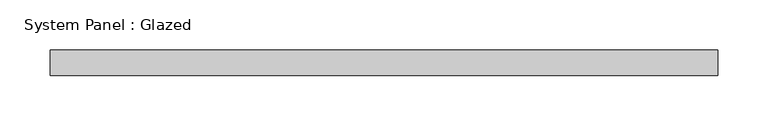
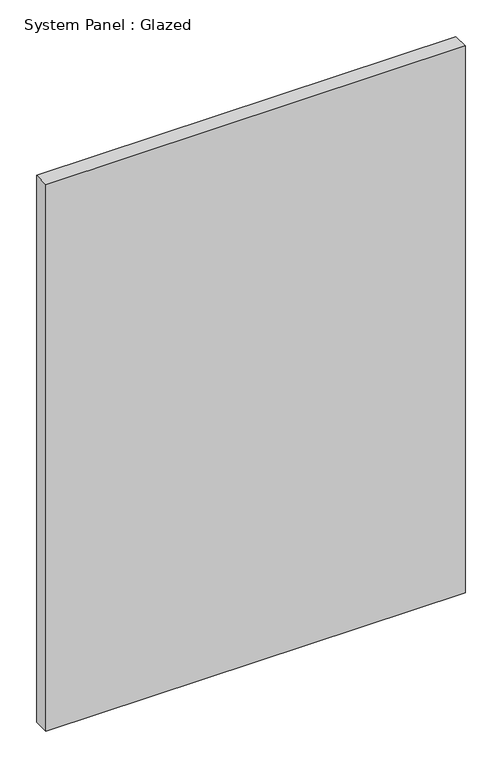
"""IFC4 building model written with IfcOpenShell, lengths in millimetres: plate geometry, System Panel : Glazed."""

from ifc_helpers import new_model, si_unit, origin, origin_with_axes, place, context, project, spatial, polyline, outline, extrude, source, transform, mapped, element, save


def system_panel_glazed_2c748f7c(model_context):
    return source(origin(), model_context, "Body", "SweptSolid", [
        extrude(outline(polyline([(331.7136159, 19.05), (-331.7136159, 19.05), (-331.7136159, 44.45), (331.7136159, 44.45), (331.7136159, 19.05)])), origin_with_axes(), (0.0, 0.0, 1.0), 914.4),
    ])


if __name__ == "__main__":
    model = new_model("IFC4")
    model_context = context("Model", 3, world=origin())
    ifc_project = project(units=[si_unit("LENGTHUNIT", "METRE", prefix="MILLI")], contexts=[model_context])
    site = spatial("IfcSite", under=ifc_project)
    building = spatial("IfcBuilding", under=site)
    placement = place(None, origin())
    system_panel_glazed_shape = system_panel_glazed_2c748f7c(model_context)
    element("IfcPlate", 1, ObjectType="System Panel : Glazed", at=placement, inside=building, context=model_context, shape_type="MappedRepresentation", body=[
        mapped(system_panel_glazed_shape, transform((0.0, 0.0, 0.0), x_axis=(1.0, 0.0, 0.0), y_axis=(0.0, 1.0, 0.0), z_axis=(0.0, 0.0, 1.0))),
    ])
    save(model, "model.ifc")

# Revit data of these elements
# Type "System Panel : Glazed"
#   Construction Type Id = "GSP4R"
#   Analytic Construction = "1/8 in Pilkington single glazing"
#   Visual Light Transmittance = 0.9
#   Solar Heat Gain Coefficient = 0.86
#   Heat Transfer Coefficient (U) = 1.18115 BTU/(h·ft²·°F)
# Element 1 (IfcPlate, "System Panel : Glazed")
#   Materials on its faces: "Glass"
# Materials
#   "Glass": class "Glass", colour RGB 0 128 192, transparency 0.75, Description = "Soda Lime Glass", Cost = 0
